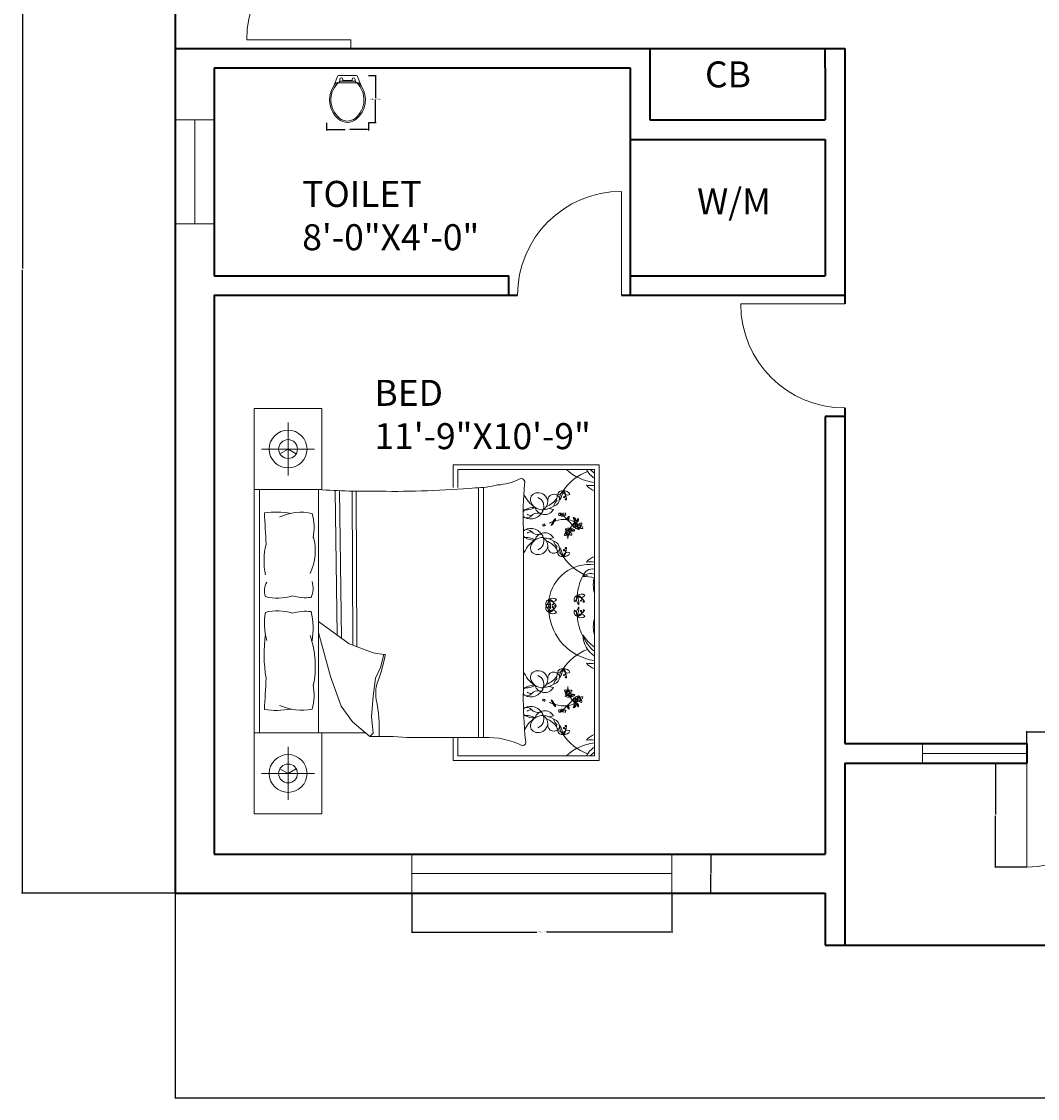
# Model space of a CAD drawing. Units: inches. Extents: x -59 to 444, y -680 to 63.
# Tile 1 of 9: x -59 to 176, y -680 to -431. Entities that reach past the tile are written whole.
import ezdxf

# ---------------------------------------------------------------- set-up
doc = ezdxf.new("R2010")
doc.units = ezdxf.units.IN
doc.header["$MEASUREMENT"] = 0
for name, color, linetype, lineweight in [('A-ANNO-DIMS', 2, 'Continuous', 18), ('A-ANNO-TEXT', 7, 'Continuous', 18), ('A-AREA-IDEN', 7, 'Continuous', 18), ('A-DOOR', 3, 'Continuous', 18), ('A-FLOR-FIXT', 9, 'Continuous', 18), ('A-FURN', 8, 'Continuous', 13), ('A-GLAZ', 4, 'Continuous', 18), ('A-WALL', 7, 'Continuous', 35)]:
    doc.layers.add(name, color=color, linetype=linetype, lineweight=lineweight)
doc.styles.get("Standard").update_dxf_attribs({"font": 'arial.ttf'})
doc.dimstyles.get("Standard").update_dxf_attribs({"dimtxt": 0.18, "dimasz": 0.18, "dimexe": 0.18, "dimexo": 0.0625, "dimgap": 0.09, "dimtad": 0, "dimtih": 1, "dimtoh": 1, "dimdec": 0, "dimzin": 0, "dimdsep": 46, "dimlunit": 3, "dimtxsty": 'Standard', "dimcen": 0.09, "dimadec": 0, "dimazin": 0, "dimtfac": 1, "dimtdec": 0, "dimtofl": 0, "dimtmove": 0, "dimatfit": 3, "dimfxl": 1, "dimtolj": 1, "dimtzin": 0, "dimarcsym": 0})

# ---------------------------------------------------------------- blocks, each defined once
blk = doc.blocks.new('BED-SET-80')
for p, q in [((0, 0), (0, 93.61)), ((7.8, 78.14), (7.8, 90.37)), ((13.92, 84.25), (1.69, 84.25)), ((45.89, 75.41), (45.89, 80.6)), ((45.89, 80.6), (79.61, 80.6)), ((79.61, 80.6), (79.61, 12.36)), ((46.97, 79.52), (46.97, 75.39)), ((78.53, 79.52), (46.97, 79.52)), ((78.53, 13.44), (78.53, 79.52)), ((1.2, 74.89), (1.2, 18.72)), ((14.79, 18.72), (14.79, 74.89)), ((18.68, 74.64), (19.15, 41.31)), ((19.64, 74.6), (20.12, 40.61)), ((51.73, 75.32), (51.73, 17.64)), ((52.89, 75.4), (52.89, 17.64)), ((22.59, 74.55), (22.73, 39.01)), ((23.55, 74.56), (23.7, 38.64)), ((69.04, 70.29), (67.98, 70.5)), ((62.09, 65.81), (62.09, 27.8)), ((69.04, 63.75), (67.98, 63.54)), ((14.79, 44.44), (21.93, 39.31)), ((17.58, 31.73), (14.79, 41.93)), ((21.93, 39.31), (27.43, 37.22)), ((27.43, 37.22), (29.89, 36.85)), ((29.89, 36.85), (29.13, 33.81)), ((29.13, 33.81), (28, 31.35)), ((20.04, 24.9), (17.58, 31.73)), ((28, 31.35), (27.43, 27.18)), ((69.04, 29.21), (67.98, 29.42)), ((22.69, 21.3), (20.04, 24.9)), ((27.43, 27.18), (27.05, 22.44)), ((27.05, 22.44), (27.43, 18.64)), ((69.04, 22.67), (67.98, 22.46)), ((26.67, 17.88), (22.69, 21.3)), ((0, 18.72), (25.69, 18.72)), ((27.43, 18.64), (26.67, 17.88)), ((45.89, 12.36), (45.89, 17.65)), ((46.97, 17.65), (46.97, 13.44)), ((7.8, 15.48), (7.8, 3.25)), ((46.97, 13.44), (78.53, 13.44)), ((79.61, 12.36), (45.89, 12.36)), ((13.92, 9.36), (1.69, 9.36))]:
    blk.add_line(p, q)
for points in [[(0, 74.89), (15.6, 74.89), (15.6, 93.61), (0, 93.61)], [(7.8, 84.25), (5.91, 83.16)], [(7.8, 84.25), (9.69, 83.16)], [(15.6, 18.72), (15.6, 0), (0, 0)], [(7.8, 9.36), (5.91, 10.45)], [(7.8, 9.36), (9.69, 10.45)]]:
    blk.add_lwpolyline(points)
for points in [[(50.99, 75.29, 0.056112), (56.14, 75.97, 0.095341), (61.1, 77.28)], [(2.33, 69.51, -0.074897), (8.45, 69.4, 0.472817)], [(8.79, 50.37, -0.14099), (2.55, 50.18, -0.235245)], [(8.79, 46.37, 0.14099), (2.55, 46.55, 0.235245)], [(2.33, 24.1, 0.074897), (8.45, 24.21, -0.472817)], [(35.24, 17.69, 0.001242), (53, 17.64, -0.127202), (61.86, 15.77)]]:
    blk.add_lwpolyline(points, format="xyb")
for centre, radius in [((7.8, 84.25), 4.37), ((7.8, 84.25), 2.18), ((72.43, 64.89), 0.238), ((74.94, 66.44), 0.238), ((72.43, 28.07), 0.238), ((74.94, 26.51), 0.238), ((7.8, 9.36), 4.37), ((7.8, 9.36), 2.18)]:
    blk.add_circle(centre, radius)
for centre, radius, start, end in [((61.58, 76.58), 0.853, 336.5219, 123.8264), ((81.38, 67.71), 12.22, 111.4092, 145.6135), ((80.17, 88.62), 12.22, 228.1144, 262.255), ((81.81, 82.49), 5.96, 209.8884, 236.5383), ((82.92, 84.63), 7.42, 223.5186, 233.6964), ((26.23, 242.71), 168.2, 266.1, 270.9282), ((32.35, 293.91), 219.42, 269.1145, 274.8735), ((153.14, 68.68), 91.09, 175.2402, 181.8035), ((71.05, 73.62), 1.01, 76.272, 177.0484), ((69.51, 75.7), 2.09, 284.7031, 328.6173), ((72.42, 73.04), 1.93, 125.7657, 194.5347), ((62.95, 76.46), 8.55, 332.8176, 347.4827), ((71.58, 73.28), 1.36, 20.9613, 102.2885), ((72.31, 74.64), 1.02, 181.7131, 301.5367), ((68.97, 72.57), 3.09, 2.0648, 41.1598), ((70.83, 73.72), 1, 316.2238, 62.3173), ((80.43, 79.15), 4.97, 221.0454, 247.4453), ((77.76, 92.77), 16.91, 266.3481, 272.5919), ((68.68, 76.7), 7.09, 203.6453, 236.3329), ((65.28, 72.57), 1.58, 88.9462, 185.5144), ((66.45, 73.05), 2.82, 193.079, 274.7067), ((65.51, 71.92), 2.24, 7.1143, 95.0551), ((64.66, 71.04), 2.17, 338.5779, 68.4181), ((65.01, 72.31), 2.72, 305.9599, 357.6409), ((66.02, 75.22), 4.42, 288.2955, 328.7386), ((69.11, 72.43), 1.4, 19.1312, 189.736), ((68.69, 72.77), 1.75, 285.6955, 4.031), ((71.02, 70.88), 1.87, 128.4175, 173.8338), ((70.63, 72.72), 0.861, 126.7319, 206.0245), ((71.41, 73.14), 0.0797, 20.2667, 316.2271), ((71.9, 72.68), 0.152, 168.5166, 2.0648), ((71.83, 72.7), 0.0737, 52.0591, 168.5166), ((10.9, 57.59), 12.07, 78.2417, 114.8684), ((63.13, 69.29), 1.13, 127.675, 162.5814), ((62.78, 74.1), 3.88, 259.249, 301.1782), ((63.79, 71.09), 2.98, 240.8249, 340.7178), ((64.47, 67.2), 3.61, 85.2696, 124.215), ((67.02, 71.45), 2.33, 196.8663, 330.0915), ((66.04, 69.98), 0.581, 254.8529, 12.6959), ((64.47, 67.2), 3.61, 53.6555, 57.2989), ((66.37, 75.26), 5.02, 273.4924, 303.7117), ((-888.54, 17.91), 892.37, 2.85022, 3.31479), ((1.24, 66.17), 12.55, 348.9631, 14.8961), ((63.13, 69.29), 1.13, 196.6343, 225.5483), ((62.9, 69.77), 1.4, 246.1646, 318.4347), ((64.33, 71.54), 2.69, 240.0851, 262.564), ((65.39, 67.57), 1.92, 74.8529, 138.4347), ((71.63, 60.26), 7.75, 110.1059, 116.9968), ((67.34, 67.64), 1.5, 336.3901, 344.4871), ((68.98, 67.25), 0.191, 83.9457, 185.6216), ((68.22, 67.43), 0.785, 328.836, 0.8141), ((68.62, 67.2), 0.449, 306.5232, 32.4668), ((69.16, 67.55), 0.191, 112.5583, 214.2343), ((69.03, 67.89), 0.449, 265.7131, 351.6568), ((68.64, 68.14), 0.785, 297.3659, 329.344), ((68.05, 68.81), 1.5, 313.6929, 321.7899), ((69.71, 67.79), 0.492, 115.5379, 168.6744), ((68.04, 68.49), 1.48, 329.344, 349.7412), ((71.63, 60.26), 7.75, 86.1723, 106.4158), ((66.86, 68.15), 2.64, 352.8698, 1.6736), ((70.36, 69.11), 0.184, 125.0752, 284.7644), ((70.64, 69.18), 0.398, 127.3642, 168.4363), ((70.33, 69.5), 0.573, 277.4968, 341.2737), ((70.78, 69.23), 0.228, 88.1325, 178.8919), ((71.24, 68.99), 0.493, 136.3462, 189.6513), ((70.96, 68.94), 0.205, 189.6513, 312.3208), ((71.01, 69.51), 0.238, 183.2768, 356.7232), ((71.76, 69.08), 0.78, 164.2829, 186.9148), ((70.84, 69.08), 0.39, 312.3208, 40.2111), ((71.66, 69.52), 0.554, 201.6382, 274.947), ((70.93, 68.76), 0.724, 42.3896, 66.5724), ((78.23, 74.49), 8.89, 217.9541, 226.8459), ((71.45, 69.18), 0.394, 10.9597, 52.2379), ((71.69, 69.15), 0.183, 274.947, 37.5263), ((72.31, 68.11), 0.191, 112.5583, 214.2343), ((72.18, 68.45), 0.449, 265.7131, 351.6568), ((71.79, 68.7), 0.785, 297.3659, 329.344), ((71.83, 64.13), 3.89, 60.7959, 85.244), ((63.55, 58.53), 12.79, 37.8256, 47.7588), ((71.2, 69.37), 1.5, 313.6929, 321.7899), ((72.86, 68.35), 0.492, 115.5379, 168.6744), ((71.19, 69.05), 1.48, 329.344, 349.7412), ((70.01, 68.71), 2.64, 352.8698, 1.6736), ((76.99, 63.73), 4.66, 130.182, 149.456), ((73.72, 68.18), 0.266, 33.0979, 123.1364), ((67.86, 64.43), 6.96, 31.1156, 34.8118), ((73.34, 67.72), 0.721, 2.3172, 70.5201), ((72.99, 66.94), 1.09, 310.9365, 22.7695), ((73.93, 67.55), 0.208, 135.7354, 318.1297), ((73.58, 67.88), 0.276, 315.7354, 31.1156), ((73.35, 67.3), 0.64, 319.3812, 5.5456), ((74.09, 67.55), 0.208, 68.2452, 250.6395), ((73.61, 67.8), 0.621, 352.6008, 57.1845), ((75.83, 63.64), 4.15, 111.7087, 116.2181), ((71.83, 64.13), 3.89, 47.5083, 55.9967), ((74.2, 67.94), 0.621, 252.8042, 349.6943), ((73.61, 66.83), 0.661, 331.1838, 51.6792), ((74.27, 68), 0.276, 248.2452, 323.6254), ((74.02, 68.16), 0.721, 291.7087, 3.0299), ((68.88, 71.96), 6.96, 323.6254, 327.3216), ((74.59, 67.98), 0.266, 325.6077, 55.6462), ((75.66, 66.51), 0.752, 121.9501, 165.2442), ((75.39, 66.95), 0.236, 44.3732, 121.9501), ((63.13, 64.75), 1.13, 134.4517, 156.7144), ((63.79, 62.95), 2.98, 19.2822, 119.1751), ((62.9, 64.27), 1.4, 41.5653, 113.8354), ((64.33, 62.5), 2.69, 97.436, 119.9149), ((65.39, 66.48), 1.92, 221.5653, 285.1471), ((67.02, 62.59), 2.33, 29.9085, 163.1337), ((66.04, 64.06), 0.581, 347.3041, 105.1471), ((66.81, 66.77), 0.293, 169.5864, 349.5616), ((66.92, 66.75), 0.18, 349.5616, 167.2949), ((67.62, 67.79), 1.48, 308.4388, 328.836), ((69.03, 66.66), 0.492, 129.5056, 182.6421), ((67.36, 69), 2.64, 296.5064, 305.3102), ((72.06, 64.56), 0.398, 93.635, 168.4363), ((72.07, 66.71), 1.09, 253.6301, 325.4631), ((72.38, 65.2), 0.769, 82.0748, 142.6895), ((72.29, 66.26), 0.79, 228.342, 274.9894), ((72.01, 65.18), 0.234, 138.2946, 276.2474), ((71.75, 64.87), 0.573, 277.4968, 341.2737), ((72.1, 65.15), 0.325, 358.5719, 143.8954), ((72.2, 64.61), 0.228, 88.1325, 178.8919), ((72.28, 65.4), 0.328, 208.8493, 269.9355), ((72.01, 65.33), 0.375, 274.2123, 318.1587), ((72.66, 64.37), 0.493, 136.3462, 189.6513), ((72.32, 66.13), 0.661, 273.8774, 357.1501), ((73.17, 64.46), 0.78, 164.2829, 186.9148), ((73.15, 64.95), 0.752, 121.9501, 165.2442), ((72.57, 66.6), 0.64, 262.0748, 308.2393), ((72.25, 64.45), 0.39, 312.3208, 40.2111), ((73.08, 64.89), 0.554, 201.6382, 274.947), ((72.63, 65.24), 0.158, 262.868, 7.094), ((72.34, 64.14), 0.724, 42.3896, 66.5724), ((72.61, 65.37), 0.47, 278.5614, 22.5914), ((72.87, 64.56), 0.394, 10.9597, 118.7804), ((76.99, 63.73), 4.66, 156.1523, 156.9499), ((72.87, 65.39), 0.236, 44.3732, 121.9501), ((73.6, 65.94), 0.661, 181.4625, 249.4747), ((73.49, 66.46), 0.64, 215.1128, 261.2773), ((74, 66.43), 1.09, 197.889, 269.722), ((73.66, 66.06), 0.79, 248.3627, 295.0101), ((73.28, 65.07), 0.769, 20.6625, 81.2773), ((74.42, 66.38), 0.769, 139.3812, 199.9959), ((73.49, 66.88), 0.79, 285.6484, 332.2957), ((74.29, 66.04), 0.184, 125.0752, 284.7644), ((74.57, 66.11), 0.398, 93.635, 168.4363), ((74.52, 66.74), 0.234, 138.2946, 276.2474), ((74.26, 66.43), 0.573, 277.4968, 341.2737), ((74.61, 66.71), 0.325, 358.5719, 143.8954), ((74.71, 66.17), 0.228, 88.1325, 178.8919), ((74.8, 66.96), 0.328, 208.8493, 269.9355), ((74.52, 66.89), 0.375, 274.2123, 318.1587), ((75.17, 65.92), 0.493, 136.3462, 189.6513), ((74.89, 65.88), 0.205, 189.6513, 312.3208), ((75.68, 66.02), 0.78, 164.2829, 186.9148), ((74.76, 66.01), 0.39, 312.3208, 40.2111), ((75.59, 66.45), 0.554, 201.6382, 274.947), ((75.14, 66.8), 0.158, 262.868, 7.094), ((74.86, 65.69), 0.724, 42.3896, 66.5724), ((75.12, 66.93), 0.47, 278.5614, 22.5914), ((75.38, 66.12), 0.394, 10.9597, 118.7804), ((75.62, 66.08), 0.183, 274.947, 37.5263), ((18.71, 58.4), 16.46, 166.3427, 191.1841), ((2.16, 60.76), 11.92, 333.8761, 16.1746), ((63.13, 64.75), 1.13, 203.2856, 232.325), ((62.78, 59.95), 3.88, 58.8218, 100.2867), ((68.68, 57.35), 7.09, 123.6671, 158.5059), ((64.47, 66.84), 3.61, 235.785, 274.7304), ((66.45, 60.99), 2.82, 85.2933, 166.921), ((64.66, 63), 2.17, 291.5819, 21.4221), ((64.47, 66.84), 3.61, 302.7011, 306.3445), ((65.01, 61.74), 2.72, 2.3591, 54.0401), ((66.37, 58.78), 5.02, 56.2883, 86.5076), ((66.02, 58.82), 4.42, 31.2614, 71.7045), ((71.02, 63.16), 1.87, 186.1662, 231.5825), ((68.69, 61.27), 1.75, 355.969, 74.3045), ((71.77, 64.48), 0.184, 125.0752, 284.7644), ((72.38, 64.32), 0.205, 189.6513, 312.3208), ((76.99, 63.73), 4.66, 175.2415, 182.8929), ((73.11, 64.52), 0.183, 274.947, 37.5263), ((65.28, 61.48), 1.58, 174.4856, 271.0538), ((65.51, 62.12), 2.24, 264.9449, 352.8857), ((69.11, 61.61), 1.4, 170.264, 340.8688), ((70.63, 61.32), 0.861, 153.9755, 233.2681), ((71.05, 60.42), 1.01, 182.9516, 283.728), ((69.51, 58.35), 2.09, 31.3827, 75.2969), ((72.42, 61), 1.93, 165.4653, 234.2343), ((62.95, 57.58), 8.55, 12.5173, 27.1824), ((68.97, 61.47), 3.09, 318.8402, 357.9352), ((70.83, 60.32), 1, 297.6827, 43.7762), ((72.31, 59.4), 1.02, 58.4633, 178.2869), ((71.58, 60.76), 1.36, 257.7115, 339.0387), ((71.46, 60.92), 0.132, 43.7762, 339.7183), ((71.9, 61.36), 0.152, 357.9352, 191.4834), ((71.83, 61.35), 0.0737, 191.4834, 307.9409), ((77.35, 48.15), 9.46, 82.8636, 171.8197), ((81.38, 66.34), 12.22, 214.3865, 248.5908), ((80.43, 54.89), 4.97, 112.5547, 138.9546), ((77.76, 41.28), 16.91, 87.4081, 93.6519), ((86.72, 49.48), 12.22, 152.5854, 175.5377), ((78.01, 54.39), 2.19, 76.3898, 169.0739), ((77.71, 52.75), 2.77, 72.8609, 131.9049), ((76.49, 49.37), 5.47, 68.117, 96.6195), ((84.95, 52.9), 6.72, 162.9798, 196.4569), ((7, 51.46), 4.63, 153.3437, 196.1026), ((8.62, 52.09), 4.96, 335.0183, 18.5407), ((11.92, 61.4), 11.47, 254.1707, 275.9871), ((68.9, 48.49), 1.36, 50.8855, 132.2127), ((74.82, 49.46), 1.01, 106.1963, 206.9726), ((72.45, 50.49), 2.09, 314.6273, 358.5415), ((76.29, 49.64), 1.93, 155.6899, 224.4589), ((75.44, 49.43), 1.36, 50.8855, 132.2127), ((75.4, 50.97), 1.02, 211.6373, 331.4609), ((73.53, 47.51), 3.09, 31.989, 71.0841), ((66.37, 47.87), 8.55, 2.7418, 17.407), ((74.57, 49.43), 1, 346.148, 92.2415), ((88.42, 50.24), 9.94, 174.3643, 175.6213), ((95.23, 45), 17.76, 160.0972, 160.2783), ((68.27, 48.52), 1.01, 106.1963, 206.9726), ((68.27, 47.56), 1.01, 153.0274, 253.8037), ((65.9, 49.55), 2.09, 314.6273, 358.5415), ((65.9, 46.53), 2.09, 1.4585, 45.3727), ((69.75, 48.7), 1.93, 155.6899, 224.4589), ((69.75, 47.38), 1.93, 135.5411, 204.3101), ((68.85, 50.03), 1.02, 211.6373, 331.4609), ((68.02, 48.5), 1, 346.148, 92.2415), ((66.98, 46.57), 3.09, 31.989, 71.0841), ((59.83, 46.94), 8.55, 2.7418, 17.407), ((59.83, 49.14), 8.55, 342.593, 357.2582), ((66.98, 49.51), 3.09, 288.9159, 328.011), ((68.02, 47.58), 1, 267.7585, 13.852), ((68.82, 48.28), 0.0797, 50.1909, 346.0209), ((68.87, 47.79), 0.132, 13.852, 309.9245), ((69.48, 48.13), 0.152, 198.4408, 31.989), ((69.4, 48.1), 0.0737, 81.9833, 198.4408), ((69.48, 47.95), 0.152, 328.011, 161.5592), ((69.4, 47.97), 0.0737, 161.5592, 278.0167), ((76.29, 46.44), 1.93, 135.5411, 204.3101), ((66.37, 48.21), 8.55, 342.593, 357.2582), ((75.36, 49.21), 0.0797, 50.1909, 346.0209), ((76.02, 49.07), 0.152, 198.4408, 31.989), ((75.95, 49.04), 0.0737, 81.9833, 198.4408), ((19.05, 44.1), 16.68, 171.5249, 193.96), ((11.92, 35.33), 11.47, 84.0129, 105.8293), ((-2.93, 42.85), 16.51, 349.8617, 13.6238), ((68.85, 46.05), 1.02, 28.5391, 148.3627), ((68.9, 47.59), 1.36, 227.7873, 309.1145), ((80.17, 47.53), 12.22, 184.4623, 262.255), ((74.82, 46.62), 1.01, 153.0274, 253.8037), ((72.45, 45.59), 2.09, 1.4585, 45.3727), ((73.53, 48.57), 3.09, 288.9159, 328.011), ((74.57, 46.65), 1, 267.7585, 13.852), ((75.4, 45.11), 1.02, 28.5391, 148.3627), ((75.44, 46.65), 1.36, 227.7873, 309.1145), ((86.72, 46.6), 12.22, 184.4623, 207.4146), ((75.41, 46.85), 0.132, 13.852, 309.9245), ((76.02, 47.01), 0.152, 328.011, 161.5592), ((75.95, 47.04), 0.0737, 161.5592, 278.0167), ((84.95, 43.18), 6.72, 163.5431, 197.0202), ((88.42, 45.84), 9.94, 184.3787, 185.6357), ((95.23, 51.08), 17.76, 199.7217, 199.9028), ((36.21, 36.93), 33.95, 172.2196, 189.497), ((-7.68, 34.04), 21.76, 348.0397, 19.2615), ((81.81, 41.4), 5.96, 181.272, 236.5383), ((85.01, 47.45), 11.04, 214.0123, 234.053), ((82.92, 43.54), 7.42, 197.8504, 233.6964), ((81.38, 26.62), 12.22, 111.4092, 145.6135), ((-5.48, 43.34), 36.3, 340.1194, 349.3383), ((29.97, 36.63), 0.226, 358.8623, 109.7536), ((68.68, 35.61), 7.09, 201.4941, 236.3329), ((65.28, 31.48), 1.58, 88.9462, 185.5144), ((65.51, 30.83), 2.24, 7.1143, 95.0551), ((69.11, 31.35), 1.4, 19.1312, 189.736), ((70.63, 31.64), 0.861, 126.7319, 206.0245), ((71.05, 32.54), 1.01, 76.272, 177.0484), ((69.51, 34.61), 2.09, 284.7031, 328.6173), ((72.42, 31.96), 1.93, 125.7657, 194.5347), ((62.95, 35.38), 8.55, 332.8176, 347.4827), ((71.58, 32.2), 1.36, 20.9613, 102.2885), ((70.83, 32.64), 1, 316.2238, 62.3173), ((68.97, 31.49), 3.09, 2.0648, 41.1598), ((72.31, 33.55), 1.02, 181.7131, 301.5367), ((77.76, 51.68), 16.91, 266.3481, 272.5919), ((80.43, 38.07), 4.97, 221.0454, 247.4453), ((-888.54, 75.7), 892.37, 356.68521, 357.14978), ((1.24, 27.44), 12.55, 345.1039, 11.0369), ((35.63, 27.93), 7.62, 156.2616, 191.3392), ((66.45, 31.97), 2.82, 193.079, 274.7067), ((64.66, 29.96), 2.17, 338.5779, 68.4181), ((65.01, 31.22), 2.72, 305.9599, 357.6409), ((66.37, 34.18), 5.02, 273.4924, 303.7117), ((66.02, 34.13), 4.42, 288.2955, 328.7386), ((68.69, 31.69), 1.75, 285.6955, 4.031), ((71.02, 29.8), 1.87, 128.4175, 173.8338), ((71.41, 32.05), 0.0797, 20.2667, 316.2271), ((71.9, 31.6), 0.152, 168.5166, 2.0648), ((71.83, 31.61), 0.0737, 52.0591, 168.5166), ((159.53, 26.69), 97.45, 179.3433, 185.6887), ((62.78, 33.01), 3.88, 259.7133, 301.1782), ((63.13, 28.21), 1.13, 127.675, 156.7144), ((63.13, 28.21), 1.13, 203.229, 225.5483), ((63.79, 30.01), 2.98, 240.8249, 340.7178), ((62.9, 28.68), 1.4, 246.1646, 318.4347), ((64.47, 26.11), 3.61, 85.2696, 124.215), ((64.33, 30.46), 2.69, 240.0851, 262.564), ((65.39, 26.48), 1.92, 74.8529, 138.4347), ((67.02, 30.37), 2.33, 196.8663, 330.0915), ((66.04, 28.9), 0.581, 254.8529, 12.6959), ((64.47, 26.11), 3.61, 53.6555, 57.2989), ((71.77, 28.47), 0.184, 75.2356, 234.9248), ((72.06, 28.4), 0.398, 191.5637, 266.365), ((72.01, 27.77), 0.234, 83.7526, 221.7054), ((72.29, 26.7), 0.79, 85.0106, 131.658), ((71.75, 28.08), 0.573, 18.7263, 82.5032), ((72.1, 27.81), 0.325, 216.1046, 1.4281), ((72.2, 28.35), 0.228, 181.1081, 271.8675), ((72.28, 27.56), 0.328, 90.0645, 151.1507), ((72.01, 27.63), 0.375, 41.8413, 85.7877), ((72.38, 28.64), 0.205, 47.6792, 170.3487), ((72.66, 28.59), 0.493, 170.3487, 223.6538), ((76.99, 29.23), 4.66, 177.1071, 184.7585), ((72.32, 26.83), 0.661, 2.8499, 86.1226), ((73.17, 28.5), 0.78, 173.0852, 195.7171), ((73.15, 28.01), 0.752, 194.7558, 238.0499), ((72.25, 28.51), 0.39, 319.7889, 47.6792), ((73.08, 28.07), 0.554, 85.053, 158.3618), ((72.63, 27.72), 0.158, 352.906, 97.132), ((72.34, 28.82), 0.724, 293.4276, 317.6104), ((72.87, 28.4), 0.394, 241.2196, 349.0403), ((72.61, 27.59), 0.47, 337.4086, 81.4386), ((76.99, 29.23), 4.66, 203.0501, 203.8477), ((72.87, 27.57), 0.236, 238.0499, 315.6268), ((73.6, 27.02), 0.661, 110.5253, 178.5375), ((74, 26.53), 1.09, 90.278, 162.111), ((73.11, 28.44), 0.183, 322.4737, 85.053), ((73.66, 26.9), 0.79, 64.9899, 111.6373), ((73.28, 27.89), 0.769, 278.7227, 339.3375), ((10.9, 36.03), 12.07, 245.1316, 281.7583), ((-6.48, 19.49), 35.33, 357.4519, 11.3392), ((66.81, 26.19), 0.293, 10.4384, 190.4136), ((66.92, 26.21), 0.18, 192.7051, 10.4384), ((71.63, 32.69), 7.75, 243.0032, 249.8941), ((67.62, 25.17), 1.48, 31.164, 51.5612), ((69.03, 26.3), 0.492, 177.3579, 230.4944), ((67.36, 23.96), 2.64, 54.6898, 63.4936), ((67.34, 25.32), 1.5, 15.5129, 23.6099), ((68.98, 25.71), 0.191, 174.3784, 276.0543), ((68.62, 25.76), 0.449, 327.5332, 53.4768), ((68.22, 25.53), 0.785, 359.1859, 31.164), ((69.16, 25.41), 0.191, 145.7657, 247.4417), ((69.03, 25.07), 0.449, 8.3432, 94.2869), ((68.64, 24.82), 0.785, 30.656, 62.6341), ((68.05, 24.15), 1.5, 38.2101, 46.3071), ((69.71, 25.17), 0.492, 191.3256, 244.4621), ((68.04, 24.47), 1.48, 10.2588, 30.656), ((71.63, 32.69), 7.75, 253.5842, 273.8277), ((66.86, 24.81), 2.64, 358.3264, 7.1302), ((78.23, 18.47), 8.89, 133.1541, 142.0459), ((72.07, 26.25), 1.09, 34.5369, 106.3699), ((72.38, 27.76), 0.769, 217.3105, 277.9252), ((72.31, 24.85), 0.191, 145.7657, 247.4417), ((63.55, 34.43), 12.79, 312.2412, 322.1744), ((71.83, 28.83), 3.89, 274.756, 299.2041), ((72.18, 24.51), 0.449, 8.3432, 94.2869), ((71.79, 24.26), 0.785, 30.656, 62.6341), ((72.57, 26.36), 0.64, 51.7607, 97.9252), ((73.49, 26.5), 0.64, 98.7227, 144.8872), ((76.99, 29.23), 4.66, 210.544, 229.818), ((73.34, 25.24), 0.721, 289.4799, 357.6828), ((67.86, 28.53), 6.96, 325.1882, 328.8844), ((74.42, 26.58), 0.769, 160.0041, 220.6188), ((72.99, 26.02), 1.09, 337.2305, 49.0635), ((73.49, 26.08), 0.79, 27.7043, 74.3516), ((73.93, 25.41), 0.208, 41.8703, 224.2646), ((73.58, 25.08), 0.276, 328.8844, 44.2646), ((73.35, 25.66), 0.64, 354.4544, 40.6188), ((74.09, 25.41), 0.208, 109.3605, 291.7548), ((73.61, 25.16), 0.621, 302.8155, 7.3992), ((75.83, 29.32), 4.15, 243.7819, 248.2913), ((71.83, 28.83), 3.89, 304.0033, 312.4917), ((73.61, 26.13), 0.661, 308.3208, 28.8162), ((74.2, 25.02), 0.621, 10.3057, 107.1958), ((74.29, 26.92), 0.184, 75.2356, 234.9248), ((74.27, 24.96), 0.276, 36.3746, 111.7548), ((74.57, 26.84), 0.398, 191.5637, 266.365), ((74.52, 26.22), 0.234, 83.7526, 221.7054), ((74.02, 24.8), 0.721, 356.9701, 68.2913), ((74.26, 26.53), 0.573, 18.7263, 82.5032), ((74.61, 26.25), 0.325, 216.1046, 1.4281), ((74.71, 26.79), 0.228, 181.1081, 271.8675), ((68.88, 21), 6.96, 32.6784, 36.3746), ((74.8, 26), 0.328, 90.0645, 151.1507), ((74.52, 26.07), 0.375, 41.8413, 85.7877), ((75.17, 27.03), 0.493, 170.3487, 223.6538), ((74.89, 27.08), 0.205, 47.6792, 170.3487), ((74.59, 24.98), 0.266, 304.3538, 34.3923), ((75.68, 26.94), 0.78, 173.0852, 195.7171), ((75.66, 26.45), 0.752, 194.7558, 238.0499), ((74.76, 26.95), 0.39, 319.7889, 47.6792), ((75.59, 26.51), 0.554, 85.053, 158.3618), ((75.14, 26.16), 0.158, 352.906, 97.132), ((74.86, 27.26), 0.724, 293.4276, 317.6104), ((75.38, 26.84), 0.394, 241.2196, 349.0403), ((75.12, 26.03), 0.47, 337.4086, 81.4386), ((75.39, 26.01), 0.236, 238.0499, 315.6268), ((75.62, 26.88), 0.183, 322.4737, 85.053), ((63.13, 23.67), 1.13, 134.4517, 153.558), ((63.13, 23.67), 1.13, 210.0293, 232.325), ((62.78, 18.86), 3.88, 58.8218, 99.1554), ((63.79, 21.87), 2.98, 19.2822, 119.1751), ((62.9, 23.19), 1.4, 41.5653, 113.8354), ((64.47, 25.76), 3.61, 235.785, 274.7304), ((64.33, 21.42), 2.69, 97.436, 119.9149), ((66.45, 19.91), 2.82, 85.2933, 166.921), ((65.39, 25.39), 1.92, 221.5653, 285.1471), ((67.02, 21.51), 2.33, 29.9085, 163.1337), ((64.66, 21.92), 2.17, 291.5819, 21.4221), ((66.04, 22.98), 0.581, 347.3041, 105.1471), ((64.47, 25.76), 3.61, 302.7011, 306.3445), ((65.01, 20.65), 2.72, 2.3591, 54.0401), ((66.37, 17.7), 5.02, 56.2883, 86.5076), ((70.36, 23.85), 0.184, 75.2356, 234.9248), ((70.64, 23.78), 0.398, 191.5637, 232.6358), ((70.33, 23.46), 0.573, 18.7263, 82.5032), ((70.78, 23.73), 0.228, 181.1081, 271.8675), ((71.24, 23.97), 0.493, 170.3487, 223.6538), ((70.96, 24.02), 0.205, 47.6792, 170.3487), ((71.01, 23.45), 0.238, 3.2768, 176.7232), ((71.76, 23.88), 0.78, 173.0852, 195.7171), ((70.84, 23.88), 0.39, 319.7889, 47.6792), ((71.66, 23.44), 0.554, 85.053, 158.3618), ((70.93, 24.2), 0.724, 293.4276, 317.6104), ((71.45, 23.78), 0.394, 307.7621, 349.0403), ((71.69, 23.81), 0.183, 322.4737, 85.053), ((71.2, 23.59), 1.5, 38.2101, 46.3071), ((72.86, 24.61), 0.492, 191.3256, 244.4621), ((71.19, 23.91), 1.48, 10.2588, 30.656), ((70.01, 24.25), 2.64, 358.3264, 7.1302), ((73.72, 24.78), 0.266, 236.8636, 326.9021), ((68.68, 16.26), 7.09, 123.6671, 153.2997), ((65.28, 20.39), 1.58, 174.4856, 271.0538), ((65.51, 21.04), 2.24, 264.9449, 352.8857), ((66.02, 17.74), 4.42, 31.2614, 71.7045), ((69.11, 20.52), 1.4, 170.264, 340.8688), ((68.69, 20.19), 1.75, 355.969, 74.3045), ((71.02, 22.08), 1.87, 186.1662, 231.5825), ((70.63, 20.24), 0.861, 153.9755, 233.2681), ((72.42, 19.92), 1.93, 165.4653, 234.2343), ((62.95, 16.5), 8.55, 12.5173, 27.1824), ((68.97, 20.38), 3.09, 318.8402, 357.9352), ((70.83, 19.24), 1, 297.6827, 43.7762), ((71.46, 19.84), 0.132, 43.7762, 339.7183), ((71.9, 20.28), 0.152, 357.9352, 191.4834), ((71.83, 20.26), 0.0737, 191.4834, 307.9409), ((29, -67.95), 85.86, 85.8294, 91.553), ((69.51, 17.26), 2.09, 31.3827, 75.2969), ((71.05, 19.33), 1.01, 182.9516, 283.728), ((72.31, 18.32), 1.02, 58.4633, 178.2869), ((71.58, 19.67), 1.36, 257.7115, 339.0387), ((81.38, 25.25), 12.22, 214.3865, 248.5908), ((80.43, 13.81), 4.97, 112.5547, 138.9546), ((61.8, 16.63), 0.864, 273.98, 27.3412), ((80.17, 4.34), 12.22, 97.745, 131.8856), ((81.81, 10.47), 5.96, 123.4617, 150.1116), ((77.76, 0.19), 16.91, 87.4081, 93.6519), ((82.92, 8.33), 7.42, 126.3036, 136.4814)]:
    blk.add_arc(centre, radius, start, end)
blk = doc.blocks.new('WC-COMPACT')
for p, q in [((1.55, 9.19), (2, 9.19)), ((2, 9.19), (4.13, 9.19)), ((6.26, 9.19), (4.13, 9.19)), ((6.26, 9.19), (6.72, 9.19))]:
    blk.add_line(p, q)
for points in [[(4.13, 10.83), (2.07, 10.83, 0.31031), (1.81, 10.65), (0.96, 8.45, 0.209071)], [(2.38, 9.52), (2.38, 9.97, -1), (3.07, 9.97), (3.07, 9.73)], [(4.13, 10.83), (6.2, 10.83, -0.31031), (6.46, 10.65), (7.3, 8.45, -0.209071)], [(5.89, 9.52), (5.89, 9.97, 1), (5.2, 9.97), (5.2, 9.73)], [(0.96, 8.45, 0.383919), (2.1, 0.78, 0.163732), (4.13, 0, 0.359733)], [(1.79, 8.97, 0.431639), (2.3, 1.03, 0.162618), (4.13, 0.32, 0.470877)], [(1.55, 9.19, 0.040937), (0.96, 8.45, 0.163732)], [(2, 9.19, 0.014165), (1.79, 8.97, 0.162618)], [(2.38, 9.52, 0.022712), (2, 9.19, 0.162618)], [(4.13, 9.52), (2.38, 9.52, 0.022712)], [(4.13, 9.52), (5.89, 9.52, -0.476108)], [(6.26, 9.19, -0.448546), (5.96, 1.03, -0.162618), (4.13, 0.32, -0.470877)], [(7.3, 8.45, -0.383919), (6.17, 0.78, -0.163732), (4.13, 0, -0.359733)], [(5.89, 9.52, -0.022712), (6.26, 9.19, -0.162618)], [(6.72, 9.19, -0.040937), (7.3, 8.45, -0.163732)]]:
    blk.add_lwpolyline(points, format="xyb")
for points in [[(5.2, 9.73), (3.07, 9.73)], [(3.07, 9.73), (3.07, 9.52)], [(5.2, 9.73), (5.2, 9.52)]]:
    blk.add_lwpolyline(points)
blk = doc.blocks.new('WIN-60-W9')
for p, q in [((60, 9), (0, 9)), ((0, 9), (0, 0)), ((60, 0), (60, 9)), ((0, 4.5), (60, 4.5)), ((0, 0), (60, 0))]:
    blk.add_line(p, q)
blk = doc.blocks.new('WIN-24-W9')
for p, q in [((0, 24), (0, 0)), ((9, 24), (0, 24)), ((4.5, 24), (4.5, 0)), ((9, 0), (9, 24)), ((0, 0), (9, 0))]:
    blk.add_line(p, q)
blk = doc.blocks.new('WIN-24-W4-5')
for p, q in [((24, 4.5), (0, 4.5)), ((0, 4.5), (0, 0)), ((24, 0), (24, 4.5)), ((24, 2.25), (0, 2.25)), ((0, 0), (24, 0))]:
    blk.add_line(p, q)
blk = doc.blocks.new('DOOR-SWING-24')
blk.add_line((24, 0), (0, 0))
blk.add_arc((24, 0), 24, 90, 180)
blk = doc.blocks.new('DOOR-DOUBLE-48')
for p, q in [((0, 0), (0, 24)), ((48, 0), (48, 24))]:
    blk.add_line(p, q)
for centre, start, end in [((0, 0), 0, 90), ((48, 0), 90, 180)]:
    blk.add_arc(centre, 24, start, end)
blk = doc.blocks.new('*D18')
at = {"layer": 'A-ANNO-DIMS', "color": 0, "lineweight": -2, "transparency": 16777216}
for p, q in [((173.23, -602.37), (173.23, -595.06)), ((173.41, -595.24), (195.74, -595.24)), ((221.05, -595.24), (198.72, -595.24)), ((221.23, -602.37), (221.23, -595.06))]:
    blk.add_line(p, q, dxfattribs=at)
at = {"layer": 'A-ANNO-DIMS', "color": 0, "transparency": 16777216}
for points in [[(173.41, -595.21), (173.41, -595.27), (173.23, -595.24)], [(221.05, -595.21), (221.05, -595.27), (221.23, -595.24)]]:
    blk.add_solid(points, dxfattribs=at)
at = {"layer": 'Defpoints', "color": 0, "transparency": 16777216}
for p in [(173.23, -595.24), (173.23, -602.44), (221.23, -602.44)]:
    blk.add_point(p, dxfattribs=at)
at = {"layer": 'A-ANNO-DIMS', "color": 0, "transparency": 16777216, "insert": (197.23, -595.24), "char_height": 0.18, "attachment_point": 5}
blk.add_mtext('\\A1;DOUBLE DOOR 48 TYP.', dxfattribs=at)
blk = doc.blocks.new('*D19')
at = {"layer": 'A-ANNO-DIMS', "color": 0, "lineweight": -2, "transparency": 16777216}
for p, q in [((173.17, -602.44), (165.85, -602.44)), ((166.03, -602.62), (166.03, -614.25)), ((166.03, -626.26), (166.03, -614.62)), ((173.17, -626.44), (165.85, -626.44))]:
    blk.add_line(p, q, dxfattribs=at)
at = {"layer": 'A-ANNO-DIMS', "color": 0, "transparency": 16777216}
for points in [[(166, -602.62), (166.06, -602.62), (166.03, -602.44)], [(166, -626.26), (166.06, -626.26), (166.03, -626.44)]]:
    blk.add_solid(points, dxfattribs=at)
at = {"layer": 'Defpoints', "color": 0, "transparency": 16777216}
for p in [(173.23, -602.44), (166.03, -626.44), (173.23, -626.44)]:
    blk.add_point(p, dxfattribs=at)
at = {"layer": 'A-ANNO-DIMS', "color": 0, "transparency": 16777216, "insert": (166.03, -614.44), "char_height": 0.18, "attachment_point": 5}
blk.add_mtext('\\A1;24 TYP.', dxfattribs=at)
blk = doc.blocks.new('*D20')
at = {"layer": 'A-ANNO-DIMS', "color": 0, "lineweight": -2, "transparency": 16777216}
for p, q in [((31.32, -632.5), (31.32, -641.62)), ((91.32, -632.5), (91.32, -641.62)), ((31.5, -641.44), (60.2, -641.44)), ((91.14, -641.44), (62.44, -641.44))]:
    blk.add_line(p, q, dxfattribs=at)
at = {"layer": 'A-ANNO-DIMS', "color": 0, "transparency": 16777216}
for points in [[(31.5, -641.41), (31.5, -641.47), (31.32, -641.44)], [(91.14, -641.41), (91.14, -641.47), (91.32, -641.44)]]:
    blk.add_solid(points, dxfattribs=at)
at = {"layer": 'Defpoints', "color": 0, "transparency": 16777216}
for p in [(31.32, -632.44), (91.32, -632.44), (91.32, -641.44)]:
    blk.add_point(p, dxfattribs=at)
at = {"layer": 'A-ANNO-DIMS', "color": 0, "transparency": 16777216, "insert": (61.32, -641.44), "char_height": 0.18, "attachment_point": 5}
blk.add_mtext('\\A1;WINDOW 60 TYP.', dxfattribs=at)
blk = doc.blocks.new('*D21')
at = {"layer": 'A-ANNO-DIMS', "color": 0, "lineweight": -2, "transparency": 16777216}
for p, q in [((91.38, -623.44), (100.5, -623.44)), ((100.32, -623.62), (100.32, -627.75)), ((100.32, -632.26), (100.32, -628.12)), ((91.38, -632.44), (100.5, -632.44))]:
    blk.add_line(p, q, dxfattribs=at)
at = {"layer": 'A-ANNO-DIMS', "color": 0, "transparency": 16777216}
for points in [[(100.29, -623.62), (100.35, -623.62), (100.32, -623.44)], [(100.29, -632.26), (100.35, -632.26), (100.32, -632.44)]]:
    blk.add_solid(points, dxfattribs=at)
at = {"layer": 'Defpoints', "color": 0, "transparency": 16777216}
for p in [(91.32, -623.44), (100.32, -623.44), (91.32, -632.44)]:
    blk.add_point(p, dxfattribs=at)
at = {"layer": 'A-ANNO-DIMS', "color": 0, "transparency": 16777216, "insert": (100.32, -627.94), "char_height": 0.18, "attachment_point": 5}
blk.add_mtext('\\A1;9 TYP.', dxfattribs=at)
blk = doc.blocks.new('*D32')
at = {"layer": 'A-ANNO-DIMS', "color": 0, "lineweight": -2, "transparency": 16777216}
for p, q in [((21.36, -443.73), (23.1, -443.73)), ((22.92, -443.91), (22.92, -448.96)), ((22.92, -454.38), (22.92, -449.33)), ((21.36, -454.56), (23.1, -454.56))]:
    blk.add_line(p, q, dxfattribs=at)
at = {"layer": 'A-ANNO-DIMS', "color": 0, "transparency": 16777216}
for points in [[(22.89, -443.91), (22.95, -443.91), (22.92, -443.73)], [(22.89, -454.38), (22.95, -454.38), (22.92, -454.56)]]:
    blk.add_solid(points, dxfattribs=at)
at = {"layer": 'Defpoints', "color": 0, "transparency": 16777216}
for p in [(21.3, -443.73), (22.92, -443.73), (21.3, -454.56)]:
    blk.add_point(p, dxfattribs=at)
at = {"layer": 'A-ANNO-DIMS', "color": 0, "transparency": 16777216, "insert": (22.92, -449.15), "char_height": 0.18, "attachment_point": 5}
blk.add_mtext('\\A1;COMPACT WC 11 TYP.', dxfattribs=at)
blk = doc.blocks.new('*D33')
at = {"layer": 'A-ANNO-DIMS', "color": 0, "lineweight": -2, "transparency": 16777216}
for p, q in [((11.68, -454.62), (11.68, -456.36)), ((21.3, -454.62), (21.3, -456.36)), ((11.86, -456.18), (15.97, -456.18)), ((21.12, -456.18), (17.01, -456.18))]:
    blk.add_line(p, q, dxfattribs=at)
at = {"layer": 'A-ANNO-DIMS', "color": 0, "transparency": 16777216}
for points in [[(11.86, -456.15), (11.86, -456.21), (11.68, -456.18)], [(21.12, -456.15), (21.12, -456.21), (21.3, -456.18)]]:
    blk.add_solid(points, dxfattribs=at)
at = {"layer": 'Defpoints', "color": 0, "transparency": 16777216}
for p in [(11.68, -454.56), (21.3, -454.56), (21.3, -456.18)]:
    blk.add_point(p, dxfattribs=at)
at = {"layer": 'A-ANNO-DIMS', "color": 0, "transparency": 16777216, "insert": (16.49, -456.18), "char_height": 0.18, "attachment_point": 5}
blk.add_mtext('\\A1;10 TYP.', dxfattribs=at)
blk = doc.blocks.new('*D46')
at = {"layer": 'A-ANNO-DIMS', "color": 0, "lineweight": -2, "transparency": 16777216}
for p, q in [((-23.27, -632.5), (-23.27, -679.87)), ((408.73, -632.5), (408.73, -679.87)), ((-23.09, -679.69), (192.44, -679.69)), ((408.55, -679.69), (193.02, -679.69))]:
    blk.add_line(p, q, dxfattribs=at)
at = {"layer": 'A-ANNO-DIMS', "color": 0, "transparency": 16777216}
for points in [[(-23.09, -679.66), (-23.09, -679.72), (-23.27, -679.69)], [(408.55, -679.66), (408.55, -679.72), (408.73, -679.69)]]:
    blk.add_solid(points, dxfattribs=at)
at = {"layer": 'Defpoints', "color": 0, "transparency": 16777216}
for p in [(-23.27, -632.44), (408.73, -632.44), (408.73, -679.69)]:
    blk.add_point(p, dxfattribs=at)
at = {"layer": 'A-ANNO-DIMS', "color": 0, "transparency": 16777216, "insert": (192.73, -679.69), "char_height": 0.18, "attachment_point": 5}
blk.add_mtext('\\A1;432', dxfattribs=at)
blk = doc.blocks.new('*D50')
at = {"layer": 'A-ANNO-DIMS', "color": 0, "lineweight": -2, "transparency": 16777216}
for p, q in [((-23.33, -344.44), (-58.7, -344.44)), ((-58.52, -344.62), (-58.52, -488.25)), ((-58.52, -632.26), (-58.52, -488.62)), ((-23.33, -632.44), (-58.7, -632.44))]:
    blk.add_line(p, q, dxfattribs=at)
at = {"layer": 'A-ANNO-DIMS', "color": 0, "transparency": 16777216}
for points in [[(-58.55, -344.62), (-58.49, -344.62), (-58.52, -344.44)], [(-58.55, -632.26), (-58.49, -632.26), (-58.52, -632.44)]]:
    blk.add_solid(points, dxfattribs=at)
at = {"layer": 'Defpoints', "color": 0, "transparency": 16777216}
for p in [(-23.27, -344.44), (-58.52, -632.44), (-23.27, -632.44)]:
    blk.add_point(p, dxfattribs=at)
at = {"layer": 'A-ANNO-DIMS', "color": 0, "transparency": 16777216, "insert": (-58.52, -488.44), "char_height": 0.18, "attachment_point": 5}
blk.add_mtext('\\A1;288', dxfattribs=at)

msp = doc.modelspace()

# ---------------------------------------------------------------- linework, layer by layer
at = {"layer": 'A-DOOR'}
msp.add_line((17.23, -435.44), (17.23, -437.44), dxfattribs=at)
at = {"layer": 'A-WALL'}
for p, q in [((-23.27, -344.44), (-23.27, -632.44)), ((-23.27, -437.44), (131.23, -437.44)), ((86.23, -437.44), (86.23, -453.94)), ((126.73, -441.94), (126.73, -437.44)), ((131.23, -437.44), (131.23, -496.44)), ((-14.27, -441.94), (-14.27, -489.94)), ((-14.27, -441.94), (81.73, -441.94)), ((81.73, -441.94), (81.73, -494.44)), ((126.73, -441.94), (126.73, -453.94)), ((86.23, -453.94), (126.73, -453.94)), ((81.73, -458.44), (126.73, -458.44)), ((126.73, -458.44), (126.73, -489.94)), ((-14.27, -489.94), (53.73, -489.94)), ((53.73, -494.44), (53.73, -489.94)), ((81.73, -489.94), (126.73, -489.94)), ((-14.27, -494.44), (55.73, -494.44)), ((-14.27, -494.44), (-14.27, -623.44)), ((79.73, -494.44), (131.23, -494.44)), ((131.23, -520.44), (131.23, -597.94)), ((131.23, -522.44), (126.73, -522.44)), ((126.73, -522.44), (126.73, -623.44)), ((131.23, -597.94), (173.23, -597.94)), ((173.23, -597.94), (173.23, -602.44)), ((131.23, -602.44), (173.23, -602.44)), ((131.23, -602.44), (131.23, -632.44)), ((-14.27, -623.44), (126.73, -623.44)), ((-23.27, -632.44), (126.73, -632.44)), ((126.73, -632.44), (126.73, -644.44)), ((131.23, -632.44), (131.23, -644.44)), ((126.73, -644.44), (267.73, -644.44))]:
    msp.add_line(p, q, dxfattribs=at)

# ---------------------------------------------------------------- block references
at = {"layer": 'A-DOOR'}
msp.add_blockref('DOOR-SWING-24', (-6.77, -435.44), dxfattribs=at)
at = {"layer": 'A-DOOR', "extrusion": (0, 0, -1), "zscale": -1}
for p, rotation in [((-79.73, -470.44), 270.0000000000002), ((-107.23, -496.44), 180)]:
    msp.add_blockref('DOOR-SWING-24', p, dxfattribs=dict(at, rotation=rotation))
at = {"layer": 'A-DOOR', "rotation": 180}
msp.add_blockref('DOOR-DOUBLE-48', (221.23, -602.44), dxfattribs=at)
at = {"layer": 'A-FLOR-FIXT'}
msp.add_blockref('WC-COMPACT', (12.35, -454.56), dxfattribs=at)
at = {"layer": 'A-FURN'}
msp.add_blockref('BED-SET-80', (-5.02, -614.19), dxfattribs=at)
at = {"layer": 'A-GLAZ', "rotation": 180}
for name, p in [('WIN-24-W9', (-14.27, -453.94)), ('WIN-24-W4-5', (173.2, -597.94))]:
    msp.add_blockref(name, p, dxfattribs=at)
at = {"layer": 'A-GLAZ'}
msp.add_blockref('WIN-60-W9', (31.32, -632.43), dxfattribs=at)

# ---------------------------------------------------------------- texts
at = {"layer": 'A-ANNO-TEXT', "char_height": 6, "attachment_point": 1}
for s, insert in [('CB', (98.99, -440.44)), ('W/M', (97.17, -469.75))]:
    msp.add_mtext(s, dxfattribs=dict(at, insert=insert))
at = {"layer": 'A-AREA-IDEN', "char_height": 6, "attachment_point": 1}
for s, insert in [('TOILET\\P8\'-0"X4\'-0"', (6.05, -468.03)), ('BED\\P11\'-9"X10\'-9"', (22.7, -513.96))]:
    msp.add_mtext(s, dxfattribs=dict(at, insert=insert))

# ---------------------------------------------------------------- dimensions: what is measured, and where the dimension line sits
at = {"layer": 'A-ANNO-DIMS'}
dim = msp.add_linear_dim(base=(-58.52, -632.44), p1=(-23.27, -344.44), p2=(-23.27, -632.44), angle=90, dimstyle='Standard', override={"dimdec": 0, "dimlfac": 1, "dimrnd": 0, "dimzin": 0, "dimdsep": 46, "dimlunit": 2}, dxfattribs=at)
dim.commit()
dim.dimension.update_dxf_attribs({"geometry": '*D50', "text_midpoint": (-58.52, -488.44)})
for base, p1, p2, angle, text, picture, middle in [((22.92, -443.73), (21.3, -454.56), (21.3, -443.73), 90, 'COMPACT WC <> TYP.', '*D32', (22.92, -449.15)), ((173.23, -595.24), (221.23, -602.44), (173.23, -602.44), 180, 'DOUBLE DOOR <> TYP.', '*D18', (197.23, -595.24)), ((166.03, -626.44), (173.23, -602.44), (173.23, -626.44), 270, '<> TYP.', '*D19', (166.03, -614.44)), ((100.32, -623.44), (91.32, -632.44), (91.32, -623.44), 90, '<> TYP.', '*D21', (100.32, -627.94))]:
    dim = msp.add_linear_dim(base=base, p1=p1, p2=p2, angle=angle, text=text, dimstyle='Standard', override={"dimdec": 0, "dimlfac": 1, "dimrnd": 0, "dimzin": 0, "dimdsep": 46, "dimlunit": 2}, dxfattribs=at)
    dim.commit()
    dim.dimension.update_dxf_attribs({"geometry": picture, "text_midpoint": middle})
for base, p1, p2, text, picture, middle in [((21.3, -456.18), (11.68, -454.56), (21.3, -454.56), '<> TYP.', '*D33', (16.49, -456.18)), ((91.32, -641.44), (31.32, -632.44), (91.32, -632.44), 'WINDOW <> TYP.', '*D20', (61.32, -641.44))]:
    dim = msp.add_linear_dim(base=base, p1=p1, p2=p2, text=text, dimstyle='Standard', override={"dimdec": 0, "dimlfac": 1, "dimrnd": 0, "dimzin": 0, "dimdsep": 46, "dimlunit": 2}, dxfattribs=at)
    dim.commit()
    dim.dimension.update_dxf_attribs({"geometry": picture, "text_midpoint": middle})
dim = msp.add_linear_dim(base=(408.73, -679.69), p1=(-23.27, -632.44), p2=(408.73, -632.44), dimstyle='Standard', override={"dimdec": 0, "dimlfac": 1, "dimrnd": 0, "dimzin": 0, "dimdsep": 46, "dimlunit": 2}, dxfattribs=at)
dim.commit()
dim.dimension.update_dxf_attribs({"geometry": '*D46', "text_midpoint": (192.73, -679.69)})

doc.saveas('drawing.dxf')
